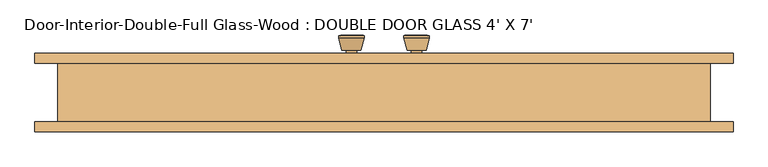
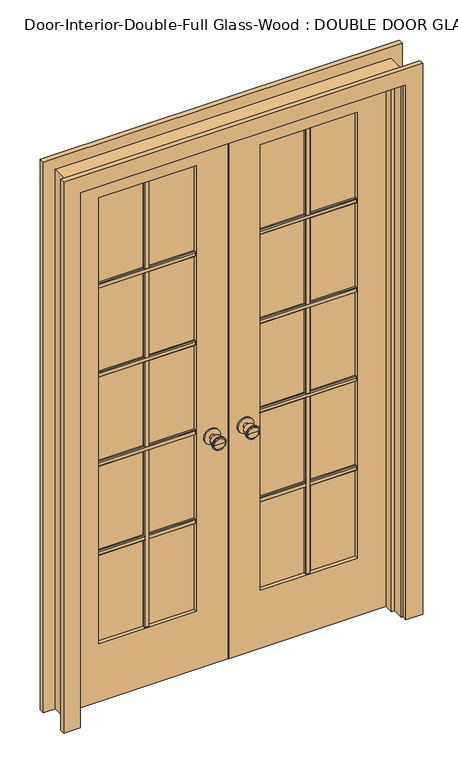
"""IFC4 building model written with IfcOpenShell, lengths in millimetres: door geometry, Door-Interior-Double-Full Glass-Wood : DOUBLE DOOR GLASS 4' X 7'."""

from ifc_helpers import new_model, si_unit, point, frame, frame_2d, origin, place, context, project, spatial, polyline, circle_curve, trimmed, segment, composite_curve, outline, extrude, faceted_brep, source, transform, mapped, element, save
from ifc_brep_helpers import plane_surface, cylinder_surface, revolved_surface, advanced_brep


def door_interior_double_full_glass_wood_double_door_glass_4_x_7_49a53587(model_context):
    return source(origin(), model_context, "Body", "SolidModel", [
        advanced_brep(
        [(-63.5, 59.975, 914.4), (-73.5, 59.975, 914.4), (-53.5, 59.975, 914.4), (-83.9758676, 108.975, 914.4), (-63.5, 108.975, 914.4), (-43.0241324, 108.975, 914.4), (-88.5, 107.1471319, 914.4), (-38.5, 107.1471319, 914.4), (-88.5, 103.6834537, 914.4), (-38.5, 103.6834537, 914.4), (-82.136236, 78.975, 914.4), (-44.863764, 78.975, 914.4), (-73.5, 78.975, 914.4), (-53.5, 78.975, 914.4)],
        [
            (0, 1),
            (1, 2, circle_curve(frame((-63.5, 59.975, 914.4), z_axis=(0.0, -1.0, 0.0), x_axis=(1.0, 0.0, 0.0)), 10.0)),
            (2, 0),
            (2, 1, circle_curve(frame((-63.5, 59.975, 914.4), z_axis=(0.0, -1.0, 0.0), x_axis=(1.0, 0.0, 0.0)), 10.0)),
            (3, 4),
            (4, 5),
            (5, 3, circle_curve(frame((-63.5, 108.975, 914.4), z_axis=(0.0, 1.0, 0.0), x_axis=(1.0, 0.0, 0.0)), 20.4758676)),
            (3, 5, circle_curve(frame((-63.5, 108.975, 914.4), z_axis=(0.0, 1.0, 0.0), x_axis=(1.0, 0.0, 0.0)), 20.4758676)),
            (6, 3),
            (5, 7),
            (7, 6, circle_curve(frame((-63.5, 107.1471319, 914.4), z_axis=(0.0, 1.0, 0.0), x_axis=(1.0, 0.0, 0.0)), 25.0)),
            (6, 7, circle_curve(frame((-63.5, 107.1471319, 914.4), z_axis=(0.0, 1.0, 0.0), x_axis=(1.0, 0.0, 0.0)), 25.0)),
            (8, 6),
            (7, 9),
            (9, 8, circle_curve(frame((-63.5, 103.6834537, 914.4), z_axis=(0.0, 1.0, 0.0), x_axis=(1.0, 0.0, 0.0)), 25.0)),
            (8, 9, circle_curve(frame((-63.5, 103.6834537, 914.4), z_axis=(0.0, 1.0, 0.0), x_axis=(1.0, 0.0, 0.0)), 25.0)),
            (10, 8),
            (9, 11),
            (11, 10, circle_curve(frame((-63.5, 78.975, 914.4), z_axis=(0.0, 1.0, 0.0), x_axis=(1.0, 0.0, 0.0)), 18.636236)),
            (10, 11, circle_curve(frame((-63.5, 78.975, 914.4), z_axis=(0.0, 1.0, 0.0), x_axis=(1.0, 0.0, 0.0)), 18.636236)),
            (12, 10),
            (11, 13),
            (13, 12, circle_curve(frame((-63.5, 78.975, 914.4), z_axis=(0.0, 1.0, 0.0), x_axis=(1.0, 0.0, 0.0)), 10.0)),
            (12, 13, circle_curve(frame((-63.5, 78.975, 914.4), z_axis=(0.0, 1.0, 0.0), x_axis=(1.0, 0.0, 0.0)), 10.0)),
            (1, 12),
            (13, 2),
        ],
        [
            plane_surface(frame((-63.5, 59.975, 914.4), z_axis=(0.0, -1.0, 0.0), x_axis=(1.0, 0.0, 0.0))),
            plane_surface(frame((-63.5, 108.975, 914.4), z_axis=(0.0, 1.0, 0.0), x_axis=(1.0, 0.0, 0.0))),
            revolved_surface(polyline([(-43.0241324, 108.975, 914.4), (-38.5, 107.1471319, 914.4)]), (-63.5, 59.975, 914.4), (0.0, -1.0, 0.0)),
            cylinder_surface(frame((-63.5, 59.975, 914.4), z_axis=(0.0, -1.0, 0.0), x_axis=(1.0, 0.0, 0.0)), 25.0),
            revolved_surface(polyline([(-38.5, 103.6834537, 914.4), (-44.863764, 78.975, 914.4)]), (-63.5, 59.975, 914.4), (0.0, -1.0, 0.0)),
            plane_surface(frame((-63.5, 78.975, 914.4), z_axis=(0.0, -1.0, 0.0), x_axis=(1.0, 0.0, 0.0))),
            cylinder_surface(frame((-63.5, 59.975, 914.4), z_axis=(0.0, -1.0, 0.0), x_axis=(1.0, 0.0, 0.0)), 10.0),
        ],
        [
            (0, [[1, 2, 3]]),
            (0, [[-3, 4, -1]]),
            (1, [[5, 6, 7]]),
            (1, [[-6, -5, 8]]),
            (2, [[9, -7, 10, 11]]),
            (2, [[-10, -8, -9, 12]]),
            (3, [[13, -11, 14, 15]]),
            (3, [[-14, -12, -13, 16]]),
            (4, [[17, -15, 18, 19]]),
            (4, [[-18, -16, -17, 20]]),
            (5, [[21, -19, 22, 23]]),
            (5, [[-22, -20, -21, 24]]),
            (6, [[25, -23, 26, -2]]),
            (6, [[-26, -24, -25, -4]]),
        ],
    ),
        extrude(outline(composite_curve([segment(trimmed(circle_curve(frame_2d((914.4, -63.5)), 30.0), [point((914.4, -33.5))], [point((914.4, -93.5))], False, "CARTESIAN"), True, "CONTINUOUS"), segment(trimmed(circle_curve(frame_2d((914.4, -63.5)), 30.0), [point((914.4, -93.5))], [point((914.4, -33.5))], False, "CARTESIAN"), True, "CONTINUOUS")], self_intersect=False)), frame((0.0, 53.975, 0.0), z_axis=(0.0, 1.0, 0.0), x_axis=(0.0, 0.0, 1.0)), (0.0, 0.0, 1.0), 6.0),
        advanced_brep(
        [(-63.5, 13.05, 914.4), (-53.5, 13.05, 914.4), (-73.5, 13.05, 914.4), (-83.9758676, -35.95, 914.4), (-43.0241324, -35.95, 914.4), (-63.5, -35.95, 914.4), (-88.5, -34.1221319, 914.4), (-38.5, -34.1221319, 914.4), (-88.5, -30.6584537, 914.4), (-38.5, -30.6584537, 914.4), (-82.136236, -5.95, 914.4), (-44.863764, -5.95, 914.4), (-73.5, -5.95, 914.4), (-53.5, -5.95, 914.4)],
        [
            (0, 1),
            (1, 2, circle_curve(frame((-63.5, 13.05, 914.4), z_axis=(0.0, 1.0, 0.0), x_axis=(1.0, 0.0, 0.0)), 10.0)),
            (2, 0),
            (2, 1, circle_curve(frame((-63.5, 13.05, 914.4), z_axis=(0.0, 1.0, 0.0), x_axis=(1.0, 0.0, 0.0)), 10.0)),
            (3, 4, circle_curve(frame((-63.5, -35.95, 914.4), z_axis=(0.0, -1.0, 0.0), x_axis=(1.0, 0.0, 0.0)), 20.4758676)),
            (4, 5),
            (5, 3),
            (4, 3, circle_curve(frame((-63.5, -35.95, 914.4), z_axis=(0.0, -1.0, 0.0), x_axis=(1.0, 0.0, 0.0)), 20.4758676)),
            (6, 7, circle_curve(frame((-63.5, -34.1221319, 914.4), z_axis=(0.0, -1.0, 0.0), x_axis=(1.0, 0.0, 0.0)), 25.0)),
            (7, 4),
            (3, 6),
            (7, 6, circle_curve(frame((-63.5, -34.1221319, 914.4), z_axis=(0.0, -1.0, 0.0), x_axis=(1.0, 0.0, 0.0)), 25.0)),
            (8, 9, circle_curve(frame((-63.5, -30.6584537, 914.4), z_axis=(0.0, -1.0, 0.0), x_axis=(1.0, 0.0, 0.0)), 25.0)),
            (9, 7),
            (6, 8),
            (9, 8, circle_curve(frame((-63.5, -30.6584537, 914.4), z_axis=(0.0, -1.0, 0.0), x_axis=(1.0, 0.0, 0.0)), 25.0)),
            (10, 11, circle_curve(frame((-63.5, -5.95, 914.4), z_axis=(0.0, -1.0, 0.0), x_axis=(1.0, 0.0, 0.0)), 18.636236)),
            (11, 9),
            (8, 10),
            (11, 10, circle_curve(frame((-63.5, -5.95, 914.4), z_axis=(0.0, -1.0, 0.0), x_axis=(1.0, 0.0, 0.0)), 18.636236)),
            (12, 13, circle_curve(frame((-63.5, -5.95, 914.4), z_axis=(0.0, -1.0, 0.0), x_axis=(1.0, 0.0, 0.0)), 10.0)),
            (13, 11),
            (10, 12),
            (13, 12, circle_curve(frame((-63.5, -5.95, 914.4), z_axis=(0.0, -1.0, 0.0), x_axis=(1.0, 0.0, 0.0)), 10.0)),
            (1, 13),
            (12, 2),
        ],
        [
            plane_surface(frame((-63.5, 13.05, 914.4), z_axis=(0.0, 1.0, 0.0), x_axis=(1.0, 0.0, 0.0))),
            plane_surface(frame((-63.5, -35.95, 914.4), z_axis=(0.0, -1.0, 0.0), x_axis=(1.0, 0.0, 0.0))),
            revolved_surface(polyline([(-43.0241324, -35.95, 914.4), (-38.5, -34.1221319, 914.4)]), (-63.5, 13.05, 914.4), (0.0, 1.0, 0.0)),
            cylinder_surface(frame((-63.5, 13.05, 914.4), z_axis=(0.0, 1.0, 0.0), x_axis=(1.0, 0.0, 0.0)), 25.0),
            revolved_surface(polyline([(-38.5, -30.6584537, 914.4), (-44.863764, -5.95, 914.4)]), (-63.5, 13.05, 914.4), (0.0, 1.0, 0.0)),
            plane_surface(frame((-63.5, -5.95, 914.4), z_axis=(0.0, 1.0, 0.0), x_axis=(1.0, 0.0, 0.0))),
            cylinder_surface(frame((-63.5, 13.05, 914.4), z_axis=(0.0, 1.0, 0.0), x_axis=(1.0, 0.0, 0.0)), 10.0),
        ],
        [
            (0, [[1, 2, 3]]),
            (0, [[-3, 4, -1]]),
            (1, [[5, 6, 7]]),
            (1, [[8, -7, -6]]),
            (2, [[9, 10, -5, 11]]),
            (2, [[12, -11, -8, -10]]),
            (3, [[13, 14, -9, 15]]),
            (3, [[16, -15, -12, -14]]),
            (4, [[17, 18, -13, 19]]),
            (4, [[20, -19, -16, -18]]),
            (5, [[21, 22, -17, 23]]),
            (5, [[24, -23, -20, -22]]),
            (6, [[-2, 25, -21, 26]]),
            (6, [[-4, -26, -24, -25]]),
        ],
    ),
        extrude(outline(composite_curve([segment(trimmed(circle_curve(frame_2d((914.4, -63.5)), 30.0), [point((914.4, -33.5))], [point((914.4, -93.5))], False, "CARTESIAN"), True, "CONTINUOUS"), segment(trimmed(circle_curve(frame_2d((914.4, -63.5)), 30.0), [point((914.4, -93.5))], [point((914.4, -33.5))], False, "CARTESIAN"), True, "CONTINUOUS")], self_intersect=False)), frame((0.0, 13.05, 0.0), z_axis=(0.0, 1.0, 0.0), x_axis=(0.0, 0.0, 1.0)), (0.0, 0.0, 1.0), 6.0),
        extrude(outline(polyline([(33.02, 1667.51), (33.02, 1648.46), (26.67, 1648.46), (23.495, 1651.635), (23.495, 1664.335), (26.67, 1667.51), (33.02, 1667.51)])), frame((120.65, 0.0, 0.0), z_axis=(1.0, 0.0, 0.0), x_axis=(0.0, 1.0, 0.0)), (0.0, 0.0, 1.0), 368.3),
        extrude(outline(polyline([(33.02, 1310.9575), (33.02, 1291.9075), (26.67, 1291.9075), (23.495, 1295.0825), (23.495, 1307.7825), (26.67, 1310.9575), (33.02, 1310.9575)])), frame((120.65, 0.0, 0.0), z_axis=(1.0, 0.0, 0.0), x_axis=(0.0, 1.0, 0.0)), (0.0, 0.0, 1.0), 368.3),
        extrude(outline(polyline([(33.02, 954.405), (33.02, 935.355), (26.67, 935.355), (23.495, 938.53), (23.495, 951.23), (26.67, 954.405), (33.02, 954.405)])), frame((120.65, 0.0, 0.0), z_axis=(1.0, 0.0, 0.0), x_axis=(0.0, 1.0, 0.0)), (0.0, 0.0, 1.0), 368.3),
        extrude(outline(polyline([(295.275, 33.02), (314.325, 33.02), (314.325, 26.67), (311.15, 23.495), (298.45, 23.495), (295.275, 26.67), (295.275, 33.02)])), frame((0.0, 0.0, 231.775), z_axis=(0.0, 0.0, 1.0), x_axis=(1.0, 0.0, 0.0)), (0.0, 0.0, 1.0), 1782.7625),
        extrude(outline(polyline([(33.02, 597.8525), (33.02, 578.8025), (26.67, 578.8025), (23.495, 581.9775), (23.495, 594.6775), (26.67, 597.8525), (33.02, 597.8525)])), frame((120.65, 0.0, 0.0), z_axis=(1.0, 0.0, 0.0), x_axis=(0.0, 1.0, 0.0)), (0.0, 0.0, 1.0), 368.3),
        extrude(outline(polyline([(40.005, 1667.51), (46.355, 1667.51), (49.53, 1664.335), (49.53, 1651.635), (46.355, 1648.46), (40.005, 1648.46), (40.005, 1667.51)])), frame((-488.95, 0.0, 0.0), z_axis=(1.0, 0.0, 0.0), x_axis=(0.0, 1.0, 0.0)), (0.0, 0.0, 1.0), 368.3),
        extrude(outline(polyline([(40.005, 1310.9575), (46.355, 1310.9575), (49.53, 1307.7825), (49.53, 1295.0825), (46.355, 1291.9075), (40.005, 1291.9075), (40.005, 1310.9575)])), frame((-488.95, 0.0, 0.0), z_axis=(1.0, 0.0, 0.0), x_axis=(0.0, 1.0, 0.0)), (0.0, 0.0, 1.0), 368.3),
        extrude(outline(polyline([(40.005, 954.405), (46.355, 954.405), (49.53, 951.23), (49.53, 938.53), (46.355, 935.355), (40.005, 935.355), (40.005, 954.405)])), frame((-488.95, 0.0, 0.0), z_axis=(1.0, 0.0, 0.0), x_axis=(0.0, 1.0, 0.0)), (0.0, 0.0, 1.0), 368.3),
        extrude(outline(polyline([(-314.325, 40.005), (-314.325, 46.355), (-311.15, 49.53), (-298.45, 49.53), (-295.275, 46.355), (-295.275, 40.005), (-314.325, 40.005)])), frame((0.0, 0.0, 231.775), z_axis=(0.0, 0.0, 1.0), x_axis=(1.0, 0.0, 0.0)), (0.0, 0.0, 1.0), 1782.7625),
        extrude(outline(polyline([(40.005, 597.8525), (46.355, 597.8525), (49.53, 594.6775), (49.53, 581.9775), (46.355, 578.8025), (40.005, 578.8025), (40.005, 597.8525)])), frame((-488.95, 0.0, 0.0), z_axis=(1.0, 0.0, 0.0), x_axis=(0.0, 1.0, 0.0)), (0.0, 0.0, 1.0), 368.3),
        extrude(outline(polyline([(40.005, 1667.51), (46.355, 1667.51), (49.53, 1664.335), (49.53, 1651.635), (46.355, 1648.46), (40.005, 1648.46), (40.005, 1667.51)])), frame((120.65, 0.0, 0.0), z_axis=(1.0, 0.0, 0.0), x_axis=(0.0, 1.0, 0.0)), (0.0, 0.0, 1.0), 368.3),
        extrude(outline(polyline([(40.005, 1310.9575), (46.355, 1310.9575), (49.53, 1307.7825), (49.53, 1295.0825), (46.355, 1291.9075), (40.005, 1291.9075), (40.005, 1310.9575)])), frame((120.65, 0.0, 0.0), z_axis=(1.0, 0.0, 0.0), x_axis=(0.0, 1.0, 0.0)), (0.0, 0.0, 1.0), 368.3),
        extrude(outline(polyline([(40.005, 954.405), (46.355, 954.405), (49.53, 951.23), (49.53, 938.53), (46.355, 935.355), (40.005, 935.355), (40.005, 954.405)])), frame((120.65, 0.0, 0.0), z_axis=(1.0, 0.0, 0.0), x_axis=(0.0, 1.0, 0.0)), (0.0, 0.0, 1.0), 368.3),
        extrude(outline(polyline([(295.275, 40.005), (295.275, 46.355), (298.45, 49.53), (311.15, 49.53), (314.325, 46.355), (314.325, 40.005), (295.275, 40.005)])), frame((0.0, 0.0, 231.775), z_axis=(0.0, 0.0, 1.0), x_axis=(1.0, 0.0, 0.0)), (0.0, 0.0, 1.0), 1782.7625),
        extrude(outline(polyline([(40.005, 597.8525), (46.355, 597.8525), (49.53, 594.6775), (49.53, 581.9775), (46.355, 578.8025), (40.005, 578.8025), (40.005, 597.8525)])), frame((120.65, 0.0, 0.0), z_axis=(1.0, 0.0, 0.0), x_axis=(0.0, 1.0, 0.0)), (0.0, 0.0, 1.0), 368.3),
        extrude(outline(polyline([(33.02, 1667.51), (33.02, 1648.46), (26.67, 1648.46), (23.495, 1651.635), (23.495, 1664.335), (26.67, 1667.51), (33.02, 1667.51)])), frame((-488.95, 0.0, 0.0), z_axis=(1.0, 0.0, 0.0), x_axis=(0.0, 1.0, 0.0)), (0.0, 0.0, 1.0), 368.3),
        extrude(outline(polyline([(33.02, 1310.9575), (33.02, 1291.9075), (26.67, 1291.9075), (23.495, 1295.0825), (23.495, 1307.7825), (26.67, 1310.9575), (33.02, 1310.9575)])), frame((-488.95, 0.0, 0.0), z_axis=(1.0, 0.0, 0.0), x_axis=(0.0, 1.0, 0.0)), (0.0, 0.0, 1.0), 368.3),
        extrude(outline(polyline([(33.02, 954.405), (33.02, 935.355), (26.67, 935.355), (23.495, 938.53), (23.495, 951.23), (26.67, 954.405), (33.02, 954.405)])), frame((-488.95, 0.0, 0.0), z_axis=(1.0, 0.0, 0.0), x_axis=(0.0, 1.0, 0.0)), (0.0, 0.0, 1.0), 368.3),
        extrude(outline(polyline([(-314.325, 33.02), (-295.275, 33.02), (-295.275, 26.67), (-298.45, 23.495), (-311.15, 23.495), (-314.325, 26.67), (-314.325, 33.02)])), frame((0.0, 0.0, 231.775), z_axis=(0.0, 0.0, 1.0), x_axis=(1.0, 0.0, 0.0)), (0.0, 0.0, 1.0), 1782.7625),
        extrude(outline(polyline([(33.02, 597.8525), (33.02, 578.8025), (26.67, 578.8025), (23.495, 581.9775), (23.495, 594.6775), (26.67, 597.8525), (33.02, 597.8525)])), frame((-488.95, 0.0, 0.0), z_axis=(1.0, 0.0, 0.0), x_axis=(0.0, 1.0, 0.0)), (0.0, 0.0, 1.0), 368.3),
        advanced_brep(
        [(63.5, 13.05, 914.4), (73.5, 13.05, 914.4), (53.5, 13.05, 914.4), (83.9758676, -35.95, 914.4), (63.5, -35.95, 914.4), (43.0241324, -35.95, 914.4), (88.5, -34.1221319, 914.4), (38.5, -34.1221319, 914.4), (88.5, -30.6584537, 914.4), (38.5, -30.6584537, 914.4), (82.136236, -5.95, 914.4), (44.863764, -5.95, 914.4), (73.5, -5.95, 914.4), (53.5, -5.95, 914.4)],
        [
            (0, 1),
            (1, 2, circle_curve(frame((63.5, 13.05, 914.4), z_axis=(0.0, 1.0, 0.0), x_axis=(-1.0, 0.0, 0.0)), 10.0)),
            (2, 0),
            (2, 1, circle_curve(frame((63.5, 13.05, 914.4), z_axis=(0.0, 1.0, 0.0), x_axis=(-1.0, 0.0, 0.0)), 10.0)),
            (3, 4),
            (4, 5),
            (5, 3, circle_curve(frame((63.5, -35.95, 914.4), z_axis=(0.0, -1.0, 0.0), x_axis=(-1.0, 0.0, 0.0)), 20.4758676)),
            (3, 5, circle_curve(frame((63.5, -35.95, 914.4), z_axis=(0.0, -1.0, 0.0), x_axis=(-1.0, 0.0, 0.0)), 20.4758676)),
            (6, 3),
            (5, 7),
            (7, 6, circle_curve(frame((63.5, -34.1221319, 914.4), z_axis=(0.0, -1.0, 0.0), x_axis=(-1.0, 0.0, 0.0)), 25.0)),
            (6, 7, circle_curve(frame((63.5, -34.1221319, 914.4), z_axis=(0.0, -1.0, 0.0), x_axis=(-1.0, 0.0, 0.0)), 25.0)),
            (8, 6),
            (7, 9),
            (9, 8, circle_curve(frame((63.5, -30.6584537, 914.4), z_axis=(0.0, -1.0, 0.0), x_axis=(-1.0, 0.0, 0.0)), 25.0)),
            (8, 9, circle_curve(frame((63.5, -30.6584537, 914.4), z_axis=(0.0, -1.0, 0.0), x_axis=(-1.0, 0.0, 0.0)), 25.0)),
            (10, 8),
            (9, 11),
            (11, 10, circle_curve(frame((63.5, -5.95, 914.4), z_axis=(0.0, -1.0, 0.0), x_axis=(-1.0, 0.0, 0.0)), 18.636236)),
            (10, 11, circle_curve(frame((63.5, -5.95, 914.4), z_axis=(0.0, -1.0, 0.0), x_axis=(-1.0, 0.0, 0.0)), 18.636236)),
            (12, 10),
            (11, 13),
            (13, 12, circle_curve(frame((63.5, -5.95, 914.4), z_axis=(0.0, -1.0, 0.0), x_axis=(-1.0, 0.0, 0.0)), 10.0)),
            (12, 13, circle_curve(frame((63.5, -5.95, 914.4), z_axis=(0.0, -1.0, 0.0), x_axis=(-1.0, 0.0, 0.0)), 10.0)),
            (1, 12),
            (13, 2),
        ],
        [
            plane_surface(frame((63.5, 13.05, 914.4), z_axis=(0.0, 1.0, 0.0), x_axis=(-1.0, 0.0, 0.0))),
            plane_surface(frame((63.5, -35.95, 914.4), z_axis=(0.0, -1.0, 0.0), x_axis=(-1.0, 0.0, 0.0))),
            revolved_surface(polyline([(43.0241324, -35.95, 914.4), (38.5, -34.1221319, 914.4)]), (63.5, 13.05, 914.4), (0.0, 1.0, 0.0)),
            cylinder_surface(frame((63.5, 13.05, 914.4), z_axis=(0.0, 1.0, 0.0), x_axis=(-1.0, 0.0, 0.0)), 25.0),
            revolved_surface(polyline([(38.5, -30.6584537, 914.4), (44.863764, -5.95, 914.4)]), (63.5, 13.05, 914.4), (0.0, 1.0, 0.0)),
            plane_surface(frame((63.5, -5.95, 914.4), z_axis=(0.0, 1.0, 0.0), x_axis=(-1.0, 0.0, 0.0))),
            cylinder_surface(frame((63.5, 13.05, 914.4), z_axis=(0.0, 1.0, 0.0), x_axis=(-1.0, 0.0, 0.0)), 10.0),
        ],
        [
            (0, [[1, 2, 3]]),
            (0, [[-3, 4, -1]]),
            (1, [[5, 6, 7]]),
            (1, [[-6, -5, 8]]),
            (2, [[9, -7, 10, 11]]),
            (2, [[-10, -8, -9, 12]]),
            (3, [[13, -11, 14, 15]]),
            (3, [[-14, -12, -13, 16]]),
            (4, [[17, -15, 18, 19]]),
            (4, [[-18, -16, -17, 20]]),
            (5, [[21, -19, 22, 23]]),
            (5, [[-22, -20, -21, 24]]),
            (6, [[25, -23, 26, -2]]),
            (6, [[-26, -24, -25, -4]]),
        ],
    ),
        extrude(outline(composite_curve([segment(trimmed(circle_curve(frame_2d((914.4, 63.5)), 30.0), [point((914.4, 33.5))], [point((914.4, 93.5))], False, "CARTESIAN"), True, "CONTINUOUS"), segment(trimmed(circle_curve(frame_2d((914.4, 63.5)), 30.0), [point((914.4, 93.5))], [point((914.4, 33.5))], False, "CARTESIAN"), True, "CONTINUOUS")], self_intersect=False)), frame((0.0, 13.05, 0.0), z_axis=(0.0, 1.0, 0.0), x_axis=(0.0, 0.0, 1.0)), (0.0, 0.0, 1.0), 6.0),
        advanced_brep(
        [(63.5, 59.975, 914.4), (53.5, 59.975, 914.4), (73.5, 59.975, 914.4), (83.9758676, 108.975, 914.4), (43.0241324, 108.975, 914.4), (63.5, 108.975, 914.4), (88.5, 107.1471319, 914.4), (38.5, 107.1471319, 914.4), (88.5, 103.6834537, 914.4), (38.5, 103.6834537, 914.4), (82.136236, 78.975, 914.4), (44.863764, 78.975, 914.4), (73.5, 78.975, 914.4), (53.5, 78.975, 914.4)],
        [
            (0, 1),
            (1, 2, circle_curve(frame((63.5, 59.975, 914.4), z_axis=(0.0, -1.0, 0.0), x_axis=(-1.0, 0.0, 0.0)), 10.0)),
            (2, 0),
            (2, 1, circle_curve(frame((63.5, 59.975, 914.4), z_axis=(0.0, -1.0, 0.0), x_axis=(-1.0, 0.0, 0.0)), 10.0)),
            (3, 4, circle_curve(frame((63.5, 108.975, 914.4), z_axis=(0.0, 1.0, 0.0), x_axis=(-1.0, 0.0, 0.0)), 20.4758676)),
            (4, 5),
            (5, 3),
            (4, 3, circle_curve(frame((63.5, 108.975, 914.4), z_axis=(0.0, 1.0, 0.0), x_axis=(-1.0, 0.0, 0.0)), 20.4758676)),
            (6, 7, circle_curve(frame((63.5, 107.1471319, 914.4), z_axis=(0.0, 1.0, 0.0), x_axis=(-1.0, 0.0, 0.0)), 25.0)),
            (7, 4),
            (3, 6),
            (7, 6, circle_curve(frame((63.5, 107.1471319, 914.4), z_axis=(0.0, 1.0, 0.0), x_axis=(-1.0, 0.0, 0.0)), 25.0)),
            (8, 9, circle_curve(frame((63.5, 103.6834537, 914.4), z_axis=(0.0, 1.0, 0.0), x_axis=(-1.0, 0.0, 0.0)), 25.0)),
            (9, 7),
            (6, 8),
            (9, 8, circle_curve(frame((63.5, 103.6834537, 914.4), z_axis=(0.0, 1.0, 0.0), x_axis=(-1.0, 0.0, 0.0)), 25.0)),
            (10, 11, circle_curve(frame((63.5, 78.975, 914.4), z_axis=(0.0, 1.0, 0.0), x_axis=(-1.0, 0.0, 0.0)), 18.636236)),
            (11, 9),
            (8, 10),
            (11, 10, circle_curve(frame((63.5, 78.975, 914.4), z_axis=(0.0, 1.0, 0.0), x_axis=(-1.0, 0.0, 0.0)), 18.636236)),
            (12, 13, circle_curve(frame((63.5, 78.975, 914.4), z_axis=(0.0, 1.0, 0.0), x_axis=(-1.0, 0.0, 0.0)), 10.0)),
            (13, 11),
            (10, 12),
            (13, 12, circle_curve(frame((63.5, 78.975, 914.4), z_axis=(0.0, 1.0, 0.0), x_axis=(-1.0, 0.0, 0.0)), 10.0)),
            (1, 13),
            (12, 2),
        ],
        [
            plane_surface(frame((63.5, 59.975, 914.4), z_axis=(0.0, -1.0, 0.0), x_axis=(-1.0, 0.0, 0.0))),
            plane_surface(frame((63.5, 108.975, 914.4), z_axis=(0.0, 1.0, 0.0), x_axis=(-1.0, 0.0, 0.0))),
            revolved_surface(polyline([(43.0241324, 108.975, 914.4), (38.5, 107.1471319, 914.4)]), (63.5, 59.975, 914.4), (0.0, -1.0, 0.0)),
            cylinder_surface(frame((63.5, 59.975, 914.4), z_axis=(0.0, -1.0, 0.0), x_axis=(-1.0, 0.0, 0.0)), 25.0),
            revolved_surface(polyline([(38.5, 103.6834537, 914.4), (44.863764, 78.975, 914.4)]), (63.5, 59.975, 914.4), (0.0, -1.0, 0.0)),
            plane_surface(frame((63.5, 78.975, 914.4), z_axis=(0.0, -1.0, 0.0), x_axis=(-1.0, 0.0, 0.0))),
            cylinder_surface(frame((63.5, 59.975, 914.4), z_axis=(0.0, -1.0, 0.0), x_axis=(-1.0, 0.0, 0.0)), 10.0),
        ],
        [
            (0, [[1, 2, 3]]),
            (0, [[-3, 4, -1]]),
            (1, [[5, 6, 7]]),
            (1, [[8, -7, -6]]),
            (2, [[9, 10, -5, 11]]),
            (2, [[12, -11, -8, -10]]),
            (3, [[13, 14, -9, 15]]),
            (3, [[16, -15, -12, -14]]),
            (4, [[17, 18, -13, 19]]),
            (4, [[20, -19, -16, -18]]),
            (5, [[21, 22, -17, 23]]),
            (5, [[24, -23, -20, -22]]),
            (6, [[-2, 25, -21, 26]]),
            (6, [[-4, -26, -24, -25]]),
        ],
    ),
        extrude(outline(composite_curve([segment(trimmed(circle_curve(frame_2d((914.4, 63.5)), 30.0), [point((914.4, 33.5))], [point((914.4, 93.5))], False, "CARTESIAN"), True, "CONTINUOUS"), segment(trimmed(circle_curve(frame_2d((914.4, 63.5)), 30.0), [point((914.4, 93.5))], [point((914.4, 33.5))], False, "CARTESIAN"), True, "CONTINUOUS")], self_intersect=False)), frame((0.0, 53.975, 0.0), z_axis=(0.0, 1.0, 0.0), x_axis=(0.0, 0.0, 1.0)), (0.0, 0.0, 1.0), 6.0),
        extrude(outline(polyline([(0.0, 615.95), (0.0, 679.45), (2203.45, 679.45), (2203.45, -679.45), (0.0, -679.45), (0.0, -615.95), (2139.95, -615.95), (2139.95, 615.95), (0.0, 615.95)])), frame((0.0, -79.375, 0.0), z_axis=(0.0, 1.0, 0.0), x_axis=(0.0, 0.0, 1.0)), (0.0, 0.0, 1.0), 19.05),
        extrude(outline(polyline([(0.0, 615.95), (0.0, 679.45), (2203.45, 679.45), (2203.45, -679.45), (0.0, -679.45), (0.0, -615.95), (2139.95, -615.95), (2139.95, 615.95), (0.0, 615.95)])), frame((0.0, 53.975, 0.0), z_axis=(0.0, 1.0, 0.0), x_axis=(0.0, 0.0, 1.0)), (0.0, 0.0, 1.0), 19.05),
        faceted_brep([(635.0, 53.975, 0.0), (635.0, -60.325, 0.0), (609.6, -60.325, 0.0), (609.6, -15.875, 0.0), (596.9, -15.875, 0.0), (596.9, 19.05, 0.0), (609.6, 19.05, 0.0), (609.6, 53.975, 0.0), (635.0, 53.975, 2159.0), (635.0, -60.325, 2159.0), (-635.0, -60.325, 2159.0), (-635.0, -60.325, 0.0), (-609.6, -60.325, 0.0), (-609.6, -60.325, 2133.6), (609.6, -60.325, 2133.6), (609.6, -15.875, 2133.6), (-609.6, -15.875, 2133.6), (-609.6, -15.875, 0.0), (-596.9, -15.875, 0.0), (-596.9, -15.875, 2120.9), (596.9, -15.875, 2120.9), (596.9, 19.05, 2120.9), (1.5875, 19.05, 2120.9), (-1.6019111, 19.05, 2120.9), (-596.9, 19.05, 2120.9), (-596.9, 19.05, 0.0), (-609.6, 19.05, 0.0), (-609.6, 19.05, 2133.6), (-1.6019111, 19.05, 2133.6), (1.5875, 19.05, 2133.6), (609.6, 19.05, 2133.6), (609.6, 53.975, 2133.6), (1.5875, 53.975, 2133.6), (-1.6019111, 53.975, 2133.6), (-609.6, 53.975, 2133.6), (-609.6, 53.975, 0.0), (-635.0, 53.975, 0.0), (-635.0, 53.975, 2159.0)], [[[0, 1, 2, 3, 4, 5, 6, 7]], [[1, 0, 8, 9]], [[2, 1, 9, 10, 11, 12, 13, 14]], [[3, 2, 14, 15]], [[4, 3, 15, 16, 17, 18, 19, 20]], [[5, 4, 20, 21]], [[6, 5, 21, 22, 23, 24, 25, 26, 27, 28, 29, 30]], [[7, 6, 30, 31]], [[0, 7, 31, 32, 33, 34, 35, 36, 37, 8]], [[9, 8, 37, 10]], [[14, 13, 16, 15]], [[20, 19, 24, 23, 22, 21]], [[31, 30, 29, 28, 27, 34, 33, 32]], [[12, 11, 36, 35, 26, 25, 18, 17]], [[11, 10, 37, 36]], [[13, 12, 17, 16]], [[19, 18, 25, 24]], [[27, 26, 35, 34]]]),
        extrude(outline(polyline([(2133.6, -609.6), (0.0, -609.6), (0.0, -1.6019111), (2133.6, -1.6019111), (2133.6, -609.6)]), holes=[polyline([(231.775, -488.95), (2014.5375, -488.95), (2014.5375, -120.65), (231.775, -120.65), (231.775, -488.95)])]), frame((0.0, 19.05, 0.0), z_axis=(0.0, 1.0, 0.0), x_axis=(0.0, 0.0, 1.0)), (0.0, 0.0, 1.0), 34.925),
        extrude(outline(polyline([(0.0, 609.6), (2133.6, 609.6), (2133.6, 1.5875), (0.0, 1.5875), (0.0, 609.6)]), holes=[polyline([(2014.5375, 120.65), (2014.5375, 488.95), (231.775, 488.95), (231.775, 120.65), (2014.5375, 120.65)])]), frame((0.0, 19.05, 0.0), z_axis=(0.0, 1.0, 0.0), x_axis=(0.0, 0.0, 1.0)), (0.0, 0.0, 1.0), 34.925),
        extrude(outline(polyline([(488.95, 33.02), (120.65, 33.02), (120.65, 40.005), (488.95, 40.005), (488.95, 33.02)])), frame((0.0, 0.0, 231.775), z_axis=(0.0, 0.0, 1.0), x_axis=(1.0, 0.0, 0.0)), (0.0, 0.0, 1.0), 1782.7625),
        extrude(outline(polyline([(-120.65, 33.02), (-488.95, 33.02), (-488.95, 40.005), (-120.65, 40.005), (-120.65, 33.02)])), frame((0.0, 0.0, 231.775), z_axis=(0.0, 0.0, 1.0), x_axis=(1.0, 0.0, 0.0)), (0.0, 0.0, 1.0), 1782.7625),
    ])


if __name__ == "__main__":
    model = new_model("IFC4")
    model_context = context("Model", 3, world=origin())
    ifc_project = project(units=[si_unit("LENGTHUNIT", "METRE", prefix="MILLI")], contexts=[model_context])
    site = spatial("IfcSite", under=ifc_project)
    building = spatial("IfcBuilding", under=site)
    placement = place(None, origin())
    door_interior_double_full_glass_wood_double_door_glass_4_x_7_shape = door_interior_double_full_glass_wood_double_door_glass_4_x_7_49a53587(model_context)
    element("IfcDoor", 1, ObjectType="Door-Interior-Double-Full Glass-Wood : DOUBLE DOOR GLASS 4' X 7'", at=placement, inside=building, context=model_context, shape_type="MappedRepresentation", body=[
        mapped(door_interior_double_full_glass_wood_double_door_glass_4_x_7_shape, transform((0.0, 0.0, 0.0), x_axis=(1.0, 0.0, 0.0), y_axis=(0.0, 1.0, 0.0), z_axis=(0.0, 0.0, 1.0))),
    ])
    save(model, "model.ifc")

# Revit data of these elements
# Type "Door-Interior-Double-Full Glass-Wood : DOUBLE DOOR GLASS 4' X 7'"
#   Type Mark = "12"
#   Assembly Code = "C1020300"
#   Analytic Construction = "French door, wood frame with single glass"
#   Top Rail = 0' - 4 11/16"
#   Thickness = 0' - 1 3/8"
#   Thermal Resistance (R) = 1.0696 (h·ft²·°F)/BTU
#   Swing Angle [instance default] = 90.00°
#   Stiles = 0' - 4 3/4"
#   Rough Width = 4' - 2"
#   Rough Height = 7' - 1"
#   Panel Width = 2' - 0"
#   Height = 7' - 0"
#   Width = 4' - 0"
#   Heat Transfer Coefficient (U) = 0.9350 BTU/(h·ft²·°F)
#   Bottom Rail = 0' - 9 1/8"
#   Show Grill [instance default] = yes
#   Trim Material = Cherry
#   Panel Material = Cherry
#   Frame Material = Cherry
#   Door Handle Material = Aluminum
#   Visual Light Transmittance = 0
#   Solar Heat Gain Coefficient = 0
#   Wall Closure = (empty or 0)
#   Function = (empty or 0)
# Element 1 (IfcDoor, "Door-Interior-Double-Full Glass-Wood : DOUBLE DOOR GLASS 4' X 7'")
#   Materials on its faces: "Cherry", "Aluminum", "Glass"
# Materials
#   "Cherry": class "Wood", colour RGB 226 177 128, transparency 0, Description = "Prunus Serotina", Cost = 0
#   "Aluminum": class "Metal", colour RGB 247 247 247, transparency 0, Description = "Aluminum 6061", Cost = 0
#   "Glass": class "Glass", colour RGB 0 128 192, transparency 0.75, Description = "Soda Lime Glass", Cost = 0
